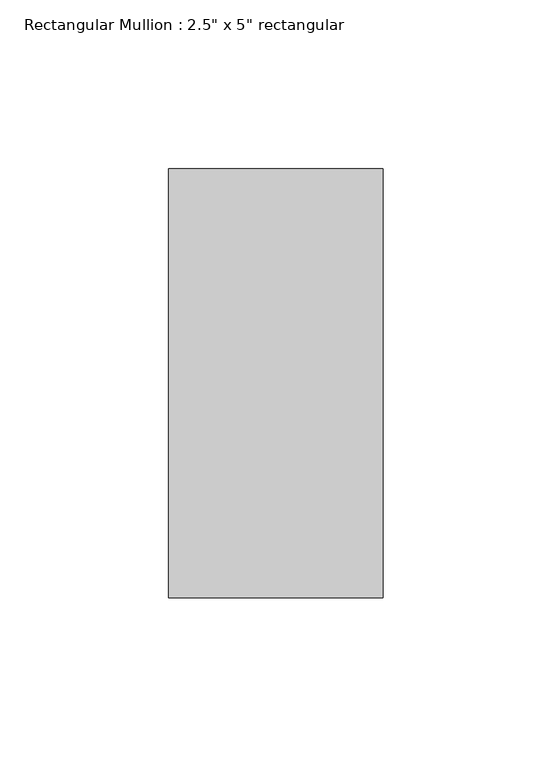
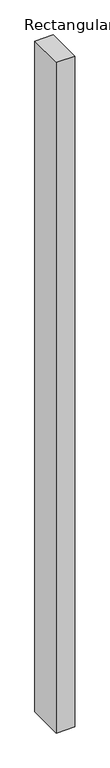
"""IFC4 building model written with IfcOpenShell, lengths in millimetres: member geometry."""

from ifc_helpers import new_model, si_unit, frame, origin, place, context, project, spatial, polyline, outline, extrude, source, transform, mapped, element, save


def member_f0fea5a5(model_context):
    return source(origin(), model_context, "Body", "SweptSolid", [
        extrude(outline(polyline([(31.75, 63.5), (31.75, -63.5), (-31.75, -63.5), (-31.75, 63.5), (31.75, 63.5)])), frame((0.0, 0.0, -2438.4), z_axis=(0.0, 0.0, 1.0), x_axis=(1.0, 0.0, 0.0)), (0.0, 0.0, 1.0), 2438.4),
    ])


if __name__ == "__main__":
    model = new_model("IFC4")
    model_context = context("Model", 3, world=origin())
    ifc_project = project(units=[si_unit("LENGTHUNIT", "METRE", prefix="MILLI")], contexts=[model_context])
    site = spatial("IfcSite", under=ifc_project)
    building = spatial("IfcBuilding", under=site)
    placement = place(None, origin())
    member_shape = member_f0fea5a5(model_context)
    element("IfcMember", 1, ObjectType="Rectangular Mullion : 2.5\" x 5\" rectangular", at=placement, inside=building, context=model_context, shape_type="MappedRepresentation", body=[
        mapped(member_shape, transform((0.0, 0.0, 0.0), x_axis=(1.0, 0.0, 0.0), y_axis=(0.0, 1.0, 0.0), z_axis=(0.0, 0.0, 1.0))),
    ])
    save(model, "model.ifc")

# Revit data of these elements
# Type "Rectangular Mullion : 2.5\" x 5\" rectangular"
#   built-in parameter 1007304 = 0.416667 (stored number, unit not read)
#   built-in parameter 1007301 = 0.104167 (stored number, unit not read)
#   built-in parameter 1007300 = 0.104167 (stored number, unit not read)
# Element 1 (IfcMember, "Rectangular Mullion : 2.5\" x 5\" rectangular")
#   Materials on its faces: "Aluminum"
# Materials
#   "Aluminum": class "Metal", colour RGB 247 247 247, transparency 0, Description = "Aluminum 6061", Cost = 0
